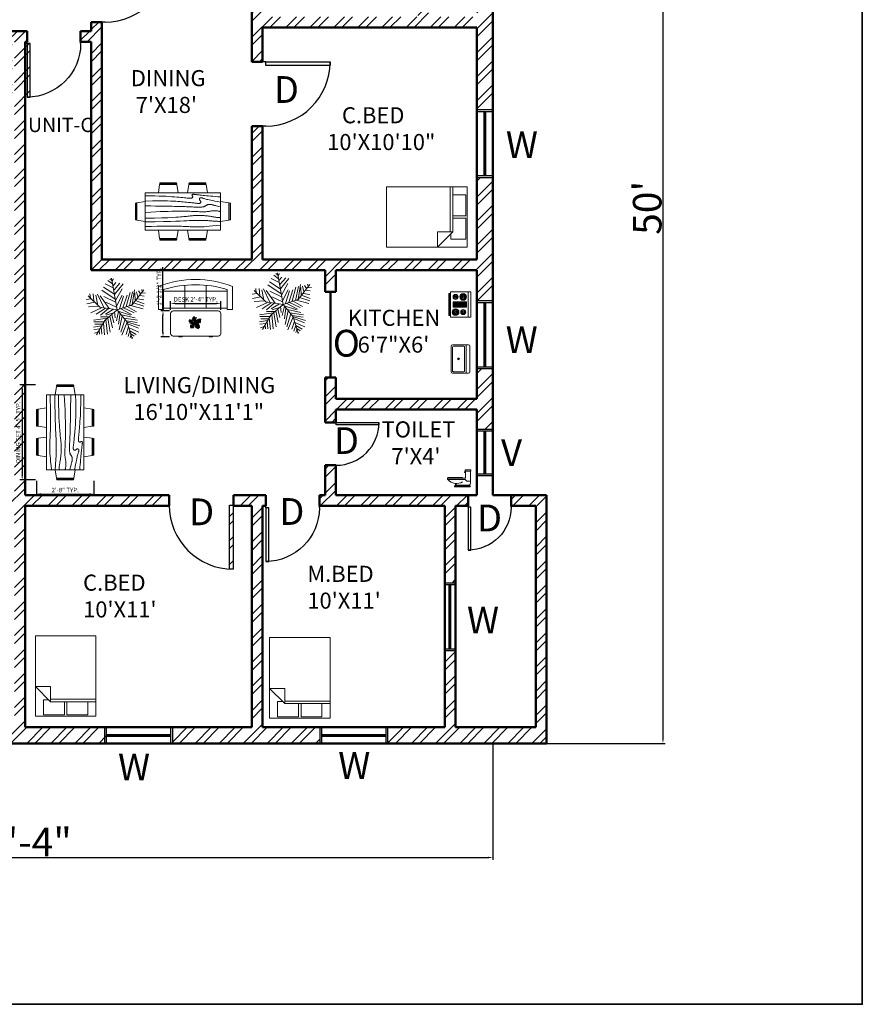
# Model space of a CAD drawing. Units: inches. Extents: x -31842 to -29388, y 18869 to 19743.
# Tile 11 of 12: x -29859 to -29388, y 18869 to 19420. Entities that reach past the tile are written whole.
import ezdxf

# ---------------------------------------------------------------- set-up
doc = ezdxf.new("R2010")
doc.units = ezdxf.units.IN
for name, color, linetype, lineweight in [('A-ANNO-DIMS', 2, 'Continuous', 18), ('A-ANNO-SYMB', 2, 'Continuous', 18), ('A-ANNO-TTLB', 7, 'Continuous', 35), ('A-AREA-IDEN', 3, 'Continuous', 18), ('A-DOOR', 3, 'Continuous', 25), ('A-FLOR-FIXT', 8, 'Continuous', 18), ('A-FURN', 8, 'Continuous', 18), ('A-GLAZ', 4, 'Continuous', 25), ('A-WALL', 7, 'Continuous', 50), ('A-WALL-PATT', 8, 'Continuous', 13), ('L-PLNT', 3, 'Continuous', 13)]:
    doc.layers.add(name, color=color, linetype=linetype, lineweight=lineweight)
doc.styles.get("Standard").update_dxf_attribs({"font": 'arial.ttf'})
doc.dimstyles.new('ISO-25', dxfattribs={"dimtxt": 2.5, "dimasz": 2.5, "dimexe": 1.25, "dimexo": 0.625, "dimtad": 1, "dimdec": 0, "dimlunit": 3, "dimtxsty": 'Standard', "dimcen": 2.5, "dimadec": 0, "dimazin": 0, "dimtfac": 1, "dimtdec": 0, "dimtmove": 0, "dimatfit": 3, "dimfxl": 1, "dimarcsym": 0})

# ---------------------------------------------------------------- blocks, each defined once
blk = doc.blocks.new('*U8')
for p, q in [((0, 0), (0, -100)), ((750, 0), (750, -100))]:
    blk.add_line(p, q)
blk.add_lwpolyline([(0, 0), (0, 750), (43.75, 750), (43.75, 0)], close=True)
blk.add_arc((0, 0), 750, 0, 90)
blk = doc.blocks.new('Bed - Queen')
for p, q in [((0, -80.00003), (0, 0)), ((0, 0), (59.99999, 0)), ((59.99999, 0), (59.99999, -80.00003)), ((7.99999, -1.2), (28.79998, -1.2)), ((7.99999, -14.4), (7.99999, -1.2)), ((28.79998, -1.2), (28.79998, -14.4)), ((31.19999, -1.2), (51.99999, -1.2)), ((31.19999, -14.4), (31.19999, -1.2)), ((51.99999, -1.2), (51.99999, -16.4)), ((0, -14.4), (44.8, -14.4)), ((44.8, -16.8), (0, -16.8)), ((59.99999, -29.6), (44.8, -14.4)), ((44.8, -14.4), (44.8, -29.6)), ((51.99999, -16.4), (46.79936, -16.4)), ((44.8, -29.6), (59.99999, -29.6)), ((59.99999, -80.00003), (0, -80.00003))]:
    blk.add_line(p, q)
blk = doc.blocks.new('Range-Oven - 30 in top')
for p, q in [((0, -3), (30, -3)), ((12, -6), (18, -6)), ((13, -20), (13, -6)), ((14, -6), (14, -20)), ((15, -20), (15, -6)), ((16, -6), (16, -20)), ((17, -20), (17, -6)), ((18, -20), (12, -20)), ((6, -24), (6, -25)), ((8, -25), (8, -24)), ((22, -25), (22, -24)), ((24, -24), (24, -25))]:
    blk.add_line(p, q)
for points in [[(0, -24), (0, 0), (30, 0), (30, -24)], [(12, -21), (12, -5), (18, -5), (18, -21)], [(2, -26), (2, -25), (28, -25), (28, -26)]]:
    blk.add_lwpolyline(points, close=True)
for centre, radius in [((6, -9), 4), ((6, -9), 3), ((6, -9), 2), ((6, -9), 1), ((24, -9), 3), ((24, -9), 2), ((24, -9), 1), ((6, -18), 3), ((6, -18), 2), ((6, -18), 1), ((24, -18), 4), ((24, -18), 3), ((24, -18), 2), ((24, -18), 1)]:
    blk.add_circle(centre, radius)
blk = doc.blocks.new('Sink-single - 30 in top')
blk.add_line((-15, -3.999996), (15, -3.999996))
for points in [[(-13.5, 0), (13.5, 0)], [(-15, -18.499996), (-15, -1.5)], [(-13.5, -17.499996), (-13.5, -6.499996)], [(-12.5, -5.499996), (12.5, -5.499996)], [(13.5, -6.499996), (13.5, -17.499996)], [(15, -1.5), (15, -18.499996)], [(13.5, -19.999996), (-13.5, -19.999996)], [(12.5, -18.499996), (-12.5, -18.499996)]]:
    blk.add_lwpolyline(points)
for radius in [1, 0.5]:
    blk.add_circle((0, -11.999996), radius)
for centre, radius, start, end in [((-13.5, -1.5), 1.5, 90, 180), ((-12.5, -6.499996), 1, 90, 180), ((12.5, -6.499996), 1, 0, 90), ((13.5, -1.5), 1.5, 0, 90), ((-13.5, -18.499996), 1.5, 180, 270), ((-12.5, -17.499996), 1, 180, 270), ((12.5, -17.499996), 1, 270, 0), ((13.5, -18.499996), 1.5, 270, 0)]:
    blk.add_arc(centre, radius, start, end)
blk = doc.blocks.new('Toilet - side')
for p, q in [((0.5, 5), (0.5, 22)), ((7.5, 22), (7.5, 12)), ((7.5, 21), (9, 21)), ((9, 20), (7.5, 20)), ((9, 21), (9, 20)), ((6, 8), (0.5, 8)), ((22, 2), (2, 2)), ((2, 2), (2, 1)), ((8, 10), (6, 8)), ((7.5, 12), (33, 12)), ((33, 10), (8, 10)), ((32.5, 13), (12, 13)), ((12, 13), (12, 12)), ((21, 4.5), (21, 2)), ((22, 2), (22, 4.5)), ((22, 1), (22, 2)), ((32.5, 12), (32.5, 13)), ((33, 12), (33, 10))]:
    blk.add_line(p, q)
for points in [[(0, 22), (0, 24), (8, 24), (8, 22)], [(1, 0), (1, 1), (23, 1), (23, 0)]]:
    blk.add_lwpolyline(points, close=True)
for centre, radius, start, end in [((3.8, 4.8), 3.26, 175.6013, 237.5288), ((20.3, 20.7), 16.2, 238.1872, 318.7702)]:
    blk.add_arc(centre, radius, start, end)
blk = doc.blocks.new('Desk - 30 x 60 in.')
for p, q in [((-26.999995, 0), (26.999995, 0)), ((-29.999995, -27), (-29.999995, -3)), ((29.999995, -3), (29.999995, -27)), ((26.999995, -30), (-26.999995, -30)), ((-20.000005, -30), (-20.000005, -31)), ((-20.000005, -31), (-16.000005, -31)), ((-16.000005, -31), (-16.000005, -30)), ((15.999995, -31), (15.999995, -30)), ((19.999995, -31), (15.999995, -31)), ((19.999995, -30), (19.999995, -31))]:
    blk.add_line(p, q)
for centre, start, end in [((-26.499995, -3.5), 98.1301, 171.8699), ((26.499995, -3.5), 8.130102, 81.8699), ((-26.499995, -26.5), 188.1301, 261.8699), ((26.499995, -26.5), 278.1301, 351.8699)]:
    blk.add_arc(centre, 3.535534, start, end)
blk = doc.blocks.new('Sofa - Roundback 7 ft.')
for p, q in [((-12.00002, -32.4421), (-12.00003, -6.5971)), ((11.99997, -32.4421), (11.99998, -6.5971)), ((-36.000027, -34), (-36.000027, -11.4696)), ((-35.999844, -13.3819), (35.9998, -13.3819)), ((35.99998, -34), (35.99998, -11.4696)), ((-36.000027, -32.4421), (35.99998, -32.4421))]:
    blk.add_line(p, q)
for points in [[(-36.000027, -34), (-42.000027, -34), (-42.000027, -8)], [(41.99998, -8), (41.99998, -34), (35.99998, -34)]]:
    blk.add_lwpolyline(points)
for centre, radius, start, end in [((0, -114.25), 114.25, 68.43141, 111.5686), ((-0.00001, -127.1968), 121.1968, 72.72033, 107.2797)]:
    blk.add_arc(centre, radius, start, end)
blk = doc.blocks.new('Dining Set - 36 x 72 in.')
for p, q in [((-22.2343, 26.00059), (-23.4847, 17.99762)), ((-22.2304, 26), (-5.7608, 26)), ((-22, 27.5), (-22.1562, 26.50042)), ((-5.8416, 26.5), (-22.1534, 26.5)), ((-22, 27.5), (-6, 27.5)), ((-5.8437, 26.49966), (-6, 27.5)), ((-4.5152, 17.99762), (-5.7655, 25.99926)), ((5.7657, 26.00059), (4.5153, 17.99762)), ((5.7696, 26), (22.2392, 26)), ((6, 27.5), (5.8438, 26.50042)), ((22.1584, 26.5), (5.8466, 26.5)), ((6, 27.5), (22, 27.5)), ((22.1563, 26.49966), (22, 27.5)), ((23.4848, 17.99762), (22.2345, 25.99926)), ((-44.0006, 8.23428), (-35.9976, 9.48474)), ((36, 18), (-36, 18)), ((-36, 18), (-36, -18)), ((44.0006, 8.23428), (35.9976, 9.48474)), ((36, -18), (36, 18)), ((-45.5, 8), (-44.5004, 8.15617)), ((-45.5, 8), (-45.5, -8)), ((-44.5, -8.15843), (-44.5, 8.15338)), ((-44, 8.23041), (-44, -8.23915)), ((44, 8.23041), (44, -8.23915)), ((44.5, -8.15843), (44.5, 8.15338)), ((45.5, 8), (44.5005, 8.15617)), ((45.5, 8), (45.5, -8)), ((-44.4997, -8.15631), (-45.5, -8)), ((-35.9976, -9.48476), (-43.9993, -8.2345)), ((35.9976, -9.48476), (43.9993, -8.2345)), ((44.4997, -8.15631), (45.5, -8)), ((-36, -18), (36, -18)), ((-22.2343, -26.0006), (-23.4847, -17.99762)), ((-4.5152, -17.99762), (-5.7655, -25.99928)), ((5.7657, -26.0006), (4.5153, -17.99762)), ((23.4848, -17.99762), (22.2345, -25.99928)), ((-22.2304, -26), (-5.7608, -26)), ((-22, -27.5), (-22.1562, -26.50044)), ((-5.8416, -26.5), (-22.1534, -26.5)), ((-22, -27.5), (-6, -27.5)), ((-5.8437, -26.49967), (-6, -27.5)), ((5.7696, -26), (22.2392, -26)), ((6, -27.5), (5.8438, -26.50044)), ((22.1584, -26.5), (5.8466, -26.5)), ((6, -27.5), (22, -27.5)), ((22.1563, -26.49967), (22, -27.5))]:
    blk.add_line(p, q)
for points in [[(-36, 15), (-31.1772, 14.97754), (-26.8079, 14.91406), (-22.8538, 14.81543), (-19.276, 14.6875), (-16.0362, 14.53613), (-13.0957, 14.36718), (-10.4159, 14.18652), (-7.9583, 14), (-5.6904, 13.81315), (-3.6035, 13.63021), (-1.6954, 13.45508), (0.0365, 13.29166), (1.5945, 13.14388), (2.9811, 13.01562), (4.1988, 12.9108), (5.25, 12.83333), (6.1393, 12.78613), (6.8802, 12.76823), (7.4883, 12.77767), (7.9792, 12.8125), (8.3685, 12.87077), (8.6719, 12.95052), (8.9049, 13.0498), (9.0833, 13.16666), (9.2205, 13.29899), (9.3216, 13.44401), (9.3895, 13.59879), (9.4271, 13.76041), (9.4373, 13.92594), (9.4232, 14.09245), (9.3875, 14.257), (9.3333, 14.41666), (9.2638, 14.56917), (9.1836, 14.71484), (9.0975, 14.85465), (9.0104, 14.98958), (8.9272, 15.1206), (8.8529, 15.2487), (8.7922, 15.37483), (8.75, 15.5), (8.7305, 15.62467), (8.7344, 15.74739), (8.7617, 15.86621), (8.8125, 15.97916), (8.8867, 16.08431), (8.9844, 16.17968), (9.1055, 16.26334), (9.25, 16.33333), (9.4189, 16.38802), (9.6172, 16.42708), (9.8506, 16.45052), (10.125, 16.45833), (10.4463, 16.45052), (10.8203, 16.42708), (11.2529, 16.38802), (11.75, 16.33333), (12.3184, 16.26318), (12.9694, 16.17838), (13.7151, 16.07991), (14.5677, 15.96875), (15.5395, 15.84586), (16.6426, 15.71224), (17.8893, 15.56884), (19.2917, 15.41666), (20.859, 15.25667), (22.5879, 15.08984), (24.4721, 14.91715), (26.5052, 14.73958), (28.6809, 14.5581), (30.9929, 14.3737), (33.4347, 14.18733), (36, 14)], [(-36, 10), (-28.9766, 10.14274), (-23.1725, 10.20442), (-18.4241, 10.19775), (-14.5677, 10.13541), (-11.4399, 10.03011), (-8.877, 9.89453), (-6.7154, 9.74137), (-4.7917, 9.58333), (-2.9698, 9.43082), (-1.2246, 9.28515), (0.4415, 9.14534), (2.026, 9.01041), (3.5266, 8.87939), (4.9408, 8.7513), (6.266, 8.62516), (7.5, 8.5), (8.6411, 8.37549), (9.6914, 8.2539), (10.6538, 8.13818), (11.5312, 8.03125), (12.3267, 7.93603), (13.043, 7.85547), (13.6831, 7.79248), (14.25, 7.75), (14.7471, 7.7303), (15.1797, 7.73307), (15.5537, 7.75732), (15.875, 7.80208), (16.1494, 7.86637), (16.3828, 7.94922), (16.5811, 8.04964), (16.75, 8.16666), (16.8944, 8.29915), (17.0143, 8.44531), (17.1089, 8.60319), (17.1771, 8.77083), (17.218, 8.94629), (17.2305, 9.1276), (17.2137, 9.31282), (17.1667, 9.5), (17.0895, 9.6875), (16.987, 9.875), (16.8649, 10.0625), (16.7292, 10.25), (16.5856, 10.4375), (16.4401, 10.625), (16.2985, 10.8125), (16.1667, 11), (16.05, 11.18733), (15.9518, 11.3737), (15.8752, 11.5581), (15.8229, 11.73958), (15.798, 11.91715), (15.8034, 12.08984), (15.842, 12.25667), (15.9167, 12.41666), (16.0295, 12.56836), (16.1784, 12.70833), (16.3605, 12.83268), (16.5729, 12.9375), (16.8127, 13.01888), (17.0768, 13.07291), (17.3625, 13.0957), (17.6667, 13.08333), (17.9894, 13.03312), (18.3418, 12.94726), (18.7382, 12.82918), (19.1927, 12.68229), (19.7195, 12.51001), (20.3327, 12.31575), (21.0465, 12.10294), (21.875, 11.875), (22.8357, 11.63354), (23.959, 11.37304), (25.2786, 11.08618), (26.8282, 10.76562), (28.6414, 10.40405), (30.752, 9.99414), (33.1936, 9.52856), (36, 9)], [(-36, 5.5), (-30.7157, 5.3348), (-26.069, 5.20963), (-21.9946, 5.11767), (-18.4271, 5.05208), (-15.3009, 5.00602), (-12.5508, 4.97265), (-10.1112, 4.94515), (-7.9167, 4.91666), (-5.909, 4.88167), (-4.0586, 4.83984), (-2.3429, 4.79215), (-0.7396, 4.73958), (0.7739, 4.6831), (2.22, 4.6237), (3.6213, 4.56233), (5, 4.5), (6.373, 4.43782), (7.7344, 4.3776), (9.0723, 4.32129), (10.375, 4.27083), (11.6309, 4.22819), (12.8281, 4.19531), (13.9551, 4.17415), (15, 4.16666), (15.954, 4.17448), (16.819, 4.19791), (17.6001, 4.23698), (18.3021, 4.29166), (18.9299, 4.36198), (19.4883, 4.44791), (19.9823, 4.54948), (20.4167, 4.66666), (20.7969, 4.79899), (21.1302, 4.94401), (21.4245, 5.09879), (21.6875, 5.26041), (21.9271, 5.42594), (22.1511, 5.59245), (22.3672, 5.757), (22.5834, 5.91666), (22.8065, 6.06868), (23.0404, 6.21093), (23.2879, 6.34147), (23.5521, 6.45833), (23.8358, 6.55957), (24.142, 6.64323), (24.4735, 6.70735), (24.8334, 6.75), (25.2235, 6.76969), (25.642, 6.76692), (26.0858, 6.74267), (26.5521, 6.69791), (27.0379, 6.63362), (27.5404, 6.55078), (28.0565, 6.45036), (28.5834, 6.33333), (29.1242, 6.19987), (29.7071, 6.04687), (30.3661, 5.87044), (31.1354, 5.66666), (32.0493, 5.43164), (33.142, 5.16146), (34.4475, 4.85221), (36, 4.5)], [(-36, -1), (-30.7915, -0.6591), (-26.0195, -0.38216), (-21.6519, -0.16284), (-17.6563, 0.00521), (-14.0005, 0.12833), (-10.6523, 0.21289), (-7.5796, 0.26522), (-4.75, 0.29166), (-2.134, 0.29793), (0.2878, 0.28711), (2.5317, 0.26163), (4.6146, 0.22396), (6.5529, 0.17651), (8.3633, 0.12174), (10.0623, 0.06209), (11.6667, 0), (13.1899, -0.06201), (14.6341, -0.1211), (15.9982, -0.17432), (17.2813, -0.21875), (18.4823, -0.25147), (19.6003, -0.26953), (20.6343, -0.27002), (21.5834, -0.25), (22.4481, -0.20768), (23.2357, -0.14584), (23.9549, -0.06836), (24.6146, 0.02083), (25.2235, 0.11784), (25.7904, 0.21875), (26.3241, 0.31966), (26.8334, 0.41666), (27.3265, 0.50618), (27.8099, 0.58593), (28.2894, 0.65397), (28.7709, 0.70833), (29.2601, 0.74707), (29.763, 0.76823), (30.2855, 0.76985), (30.8334, 0.75), (31.4088, 0.70784), (31.9994, 0.64713), (32.589, 0.57275), (33.1615, 0.48958), (33.7008, 0.4025), (34.1908, 0.3164), (34.6153, 0.23616), (34.9584, 0.16666), (35.2099, 0.11165), (35.3848, 0.07031), (35.504, 0.04069), (35.5886, 0.02083), (35.6594, 0.00879), (35.7377, 0.0026), (35.8442, 0.00032), (36, 0)], [(-36, -6.5), (-27.1843, -6.31267), (-20.084, -6.1263), (-14.469, -5.9419), (-10.1094, -5.76042), (-6.7752, -5.58285), (-4.2363, -5.41016), (-2.2629, -5.24333), (-0.625, -5.08334), (0.8708, -4.93099), (2.2715, -4.78646), (3.5872, -4.64974), (4.8281, -4.52084), (6.0046, -4.39974), (7.127, -4.28646), (8.2053, -4.18099), (9.25, -4.08334), (10.2705, -3.99382), (11.2734, -3.91407), (12.2647, -3.84603), (13.25, -3.79167), (14.2354, -3.75293), (15.2266, -3.73177), (16.2295, -3.73015), (17.25, -3.75), (18.2912, -3.79248), (19.3451, -3.85547), (20.4009, -3.93604), (21.4479, -4.03125), (22.4754, -4.13819), (23.4727, -4.25391), (24.4289, -4.37549), (25.3334, -4.5), (26.1785, -4.62492), (26.9694, -4.74935), (27.7145, -4.87281), (28.4219, -4.99479), (29.1, -5.11483), (29.7572, -5.23242), (30.4016, -5.34709), (31.0417, -5.45834), (31.6837, -5.56437), (32.3262, -5.65821), (32.9658, -5.73153), (33.599, -5.77604), (34.2224, -5.78345), (34.8327, -5.74545), (35.4264, -5.65373), (36, -5.5)], [(-36, -10), (-26.4022, -9.81299), (-18.4675, -9.62891), (-11.9839, -9.45069), (-6.7396, -9.28125), (-2.5226, -9.12354), (0.8789, -8.98047), (3.6769, -8.85498), (6.0833, -8.75), (8.2767, -8.66765), (10.3021, -8.60677), (12.1712, -8.56543), (13.8958, -8.54167), (15.4876, -8.53353), (16.9583, -8.53907), (18.3197, -8.55632), (19.5834, -8.58334), (20.7616, -8.61841), (21.8685, -8.66081), (22.9188, -8.71004), (23.9271, -8.76563), (24.9081, -8.82707), (25.8763, -8.89388), (26.8465, -8.96558), (27.8334, -9.04167), (28.8474, -9.12118), (29.8828, -9.20117), (30.93, -9.27824), (31.9792, -9.34896), (33.0205, -9.40991), (34.0443, -9.45768), (35.0407, -9.48885), (36, -9.5)], [(-36, -14.5), (-30.0881, -14.33513), (-25.0332, -14.21224), (-20.7312, -14.12647), (-17.0781, -14.07292), (-13.97, -14.04671), (-11.3027, -14.04297), (-8.9724, -14.05681), (-6.875, -14.08334), (-4.9224, -14.11833), (-3.0905, -14.16016), (-1.3709, -14.20785), (0.2448, -14.26042), (1.7647, -14.3169), (3.1973, -14.3763), (4.5507, -14.43767), (5.8333, -14.5), (7.0554, -14.5621), (8.235, -14.62175), (9.3922, -14.67652), (10.5469, -14.72396), (11.7192, -14.76164), (12.929, -14.78711), (14.1965, -14.79794), (15.5417, -14.79167), (16.9933, -14.76424), (18.6152, -14.70508), (20.4804, -14.60197), (22.6615, -14.44271), (25.2312, -14.21509), (28.2624, -13.9069), (31.8277, -13.50594), (36, -13)]]:
    blk.add_lwpolyline(points)
blk = doc.blocks.new('*U122')
for p, q in [((-258.7244, 1362.456), (-332.3336, 1421.4348)), ((0, 0), (-266.7, 1447.8)), ((-231.1146, 1315.2628), (-166.7002, 1421.4348)), ((-129.8956, 713.6638), (-626.7704, 1032.1544)), ((-185.1152, 1008.5578), (-553.1612, 1185.4942)), ((-221.9198, 1197.3052), (-433.5526, 1338.8594)), ((-194.31, 1102.9442), (-65.4812, 1256.284)), ((-148.3106, 914.1968), (118.5418, 1220.9018)), ((-129.8956, 701.8528), (265.7602, 1185.4942)), ((-74.7014, 418.7444), (219.7608, 961.39)), ((685.8, 228.6), (1219.2, 914.4)), ((689.0258, 230.0224), (790.2448, 914.1968)), ((1121.4862, 925.9824), (1149.0706, 831.6214)), ((-1206.4492, 501.3198), (-1418.082, 465.9376)), ((-800.1, 114.3), (-1333.5, 647.7)), ((-1234.059, 536.7274), (-1252.4486, 737.2604)), ((-1105.2302, 725.4494), (-1077.6458, 395.1732)), ((-976.4268, 666.4706), (-884.4026, 194.6402)), ((-902.8176, 713.6638), (-617.5756, 100.2538)), ((-369.1382, 53.086), (-783.1836, 642.874)), ((-93.091, 489.5342), (-700.3796, 902.3858)), ((-617.5756, 607.4918), (-74.7014, 347.98)), ((-28.6766, 171.0436), (228.9556, 678.2816)), ((100.1268, 41.275), (284.1498, 619.2774)), ((256.5654, 88.4682), (449.7832, 666.4706)), ((412.9786, 147.447), (587.8068, 796.2392)), ((560.197, 182.8292), (698.2206, 819.8358)), ((808.6344, 784.4282), (827.0494, 418.7444)), ((891.4384, 831.6214), (946.658, 572.1096)), ((919.0482, 501.3198), (1222.6798, 454.152)), ((983.4626, 867.0036), (1066.2666, 725.4494)), ((1029.462, 654.685), (1241.0948, 631.0884)), ((1112.2914, 760.8316), (1296.3144, 784.4282)), ((-1031.621, 347.98), (-1399.667, 277.1902)), ((-847.598, 159.2326), (-1326.0578, 135.636)), ((-718.7946, 88.4682), (-1215.644, -147.447)), ((-543.9664, 76.6572), (-967.2066, -206.4512)), ((0, 0), (-800.1, 114.3)), ((-405.9428, 53.086), (-764.794, -241.8334)), ((0, 0), (-571.5, -495.3)), ((-166.7002, 29.4894), (-543.9664, -206.4512)), ((-525.5514, 347.98), (-28.6766, 123.8504)), ((0, 0), (685.8, 228.6)), ((0, 0), (457.2, -571.5)), ((164.5412, 41.275), (661.416, -218.2368)), ((284.1498, 88.4682), (781.0246, -147.447)), ((458.978, 147.447), (891.4384, -88.4682)), ((615.4166, 194.6402), (1185.8752, 41.275)), ((753.4148, 312.5978), (1222.6798, 159.2326)), ((845.439, 418.7444), (1241.0948, 277.1902)), ((-442.7474, -383.3876), (-1086.8406, -477.7486)), ((-387.5278, -324.4088), (-764.794, -324.4088)), ((-166.7002, -147.447), (-507.1618, -253.619)), ((-433.5526, -383.3876), (-323.1134, -1020.3688)), ((-341.5284, -289.0012), (-221.9198, -831.6214)), ((-240.3094, -218.2368), (-157.5054, -595.7062)), ((-120.7008, -88.4682), (-93.091, -371.5766)), ((63.3222, -76.6826), (-37.8714, -513.1308)), ((44.9326, -64.897), (615.4166, -241.8334)), ((127.7366, -159.258), (54.1274, -654.685)), ((228.9556, -289.0012), (90.932, -914.1968)), ((357.759, -430.5554), (164.5412, -1020.3688)), ((192.151, -230.0224), (817.8292, -371.5766)), ((311.7596, -383.3876), (937.4378, -477.7486)), ((-718.7946, -737.2604), (-1086.8406, -796.2392)), ((-617.5756, -548.5384), (-1077.6458, -560.324)), ((-783.1836, -867.029), (-1077.6458, -902.4112)), ((-681.9646, -666.496), (-1022.4262, -654.685)), ((-571.5, -495.3), (-952.5, -1143)), ((-737.1842, -784.4536), (-709.5744, -1114.7298)), ((-635.9652, -607.5172), (-580.771, -1150.1374)), ((-525.5514, -465.963), (-451.9422, -1126.5408)), ((458.978, -572.1096), (210.5406, -1161.923)), ((514.1976, -772.6426), (403.7838, -1138.3264)), ((412.9786, -501.3452), (919.0482, -583.9206)), ((457.2, -571.5), (685.8, -1333.5)), ((468.1982, -572.1096), (1029.462, -737.2604)), ((486.5878, -642.8994), (983.4626, -843.4324)), ((541.8074, -831.6214), (992.6574, -1032.1544)), ((-875.2078, -1008.5832), (-1040.8412, -1079.3476)), ((-829.2084, -937.7934), (-810.7934, -1126.5408)), ((578.612, -961.39), (495.7826, -1232.7128)), ((578.612, -973.1756), (873.0488, -1138.3264)), ((624.6114, -1161.923), (587.8068, -1291.6916)), ((624.6114, -1102.9442), (781.0246, -1209.1162)), ((679.8056, -1268.095), (716.6102, -1291.6916))]:
    blk.add_line(p, q)
blk = doc.blocks.new('*D211')
at = {"layer": 'A-ANNO-DIMS', "color": 0, "lineweight": -2, "transparency": 16777216}
for p, q in [((-29593.87, 19614.96), (-29498.06, 19614.96)), ((-29499.31, 19612.46), (-29499.31, 19017.46)), ((-29593.87, 19014.96), (-29498.06, 19014.96))]:
    blk.add_line(p, q, dxfattribs=at)
at = {"layer": 'A-ANNO-DIMS', "color": 0, "transparency": 16777216}
for points in [[(-29499.72, 19612.46), (-29498.89, 19612.46), (-29499.31, 19614.96)], [(-29499.72, 19017.46), (-29498.89, 19017.46), (-29499.31, 19014.96)]]:
    blk.add_solid(points, dxfattribs=at)
at = {"layer": 'Defpoints', "color": 0, "transparency": 16777216}
for p in [(-29594.5, 19614.96), (-29594.5, 19014.96), (-29499.31, 19014.96)]:
    blk.add_point(p, dxfattribs=at)
at = {"layer": 'A-ANNO-DIMS', "color": 0, "transparency": 16777216, "insert": (-29508.1, 19314.96), "char_height": 2.5, "attachment_point": 5, "rotation": 90}
blk.add_mtext("{\\H6.4x;50'}", dxfattribs=at)
blk = doc.blocks.new('*D212')
at = {"layer": 'A-ANNO-DIMS', "color": 0, "lineweight": -2, "transparency": 16777216}
for p, q in [((-30126.5, 19014.34), (-30126.5, 18949.8)), ((-29594.5, 19014.34), (-29594.5, 18949.8)), ((-30124, 18951.05), (-29597, 18951.05))]:
    blk.add_line(p, q, dxfattribs=at)
at = {"layer": 'A-ANNO-DIMS', "color": 0, "transparency": 16777216}
for points in [[(-30124, 18951.47), (-30124, 18950.64), (-30126.5, 18951.05)], [(-29597, 18951.47), (-29597, 18950.64), (-29594.5, 18951.05)]]:
    blk.add_solid(points, dxfattribs=at)
at = {"layer": 'Defpoints', "color": 0, "transparency": 16777216}
for p in [(-30126.5, 19014.96), (-29594.5, 19014.96), (-29594.5, 18951.05)]:
    blk.add_point(p, dxfattribs=at)
at = {"layer": 'A-ANNO-DIMS', "color": 0, "transparency": 16777216, "insert": (-29860.5, 18959.68), "char_height": 2.5, "attachment_point": 5}
blk.add_mtext('{\\H6.4x;44\'-4"}', dxfattribs=at)
blk = doc.blocks.new('WIN-3FT')
for p, q in [((0, 36), (9, 36)), ((4, 0), (4, 36)), ((4.5, 0), (4.5, 36)), ((5, 0), (5, 36)), ((0, 0), (9, 0))]:
    blk.add_line(p, q)
blk = doc.blocks.new('WIN-3FT-B')
for p, q in [((0, 36), (6, 36)), ((2.5, 0), (2.5, 36)), ((3, 0), (3, 36)), ((3.5, 0), (3.5, 36)), ((0, 0), (6, 0))]:
    blk.add_line(p, q)
blk = doc.blocks.new('WIN-2FT')
for p, q in [((0, 24), (9, 24)), ((4, 0), (4, 24)), ((4.5, 0), (4.5, 24)), ((5, 0), (5, 24)), ((0, 0), (9, 0))]:
    blk.add_line(p, q)
blk = doc.blocks.new('*D245')
at = {"layer": 'A-ANNO-DIMS', "color": 0, "lineweight": -2, "transparency": 16777216}
for p, q in [((-29850.74, 19215.8), (-29859.34, 19215.8)), ((-29858.09, 19213.3), (-29858.09, 19165.11)), ((-29850.74, 19162.61), (-29859.34, 19162.61))]:
    blk.add_line(p, q, dxfattribs=at)
at = {"layer": 'A-ANNO-DIMS', "color": 0, "transparency": 16777216}
for points in [[(-29858.51, 19213.3), (-29857.67, 19213.3), (-29858.09, 19215.8)], [(-29858.51, 19165.11), (-29857.67, 19165.11), (-29858.09, 19162.61)]]:
    blk.add_solid(points, dxfattribs=at)
at = {"layer": 'Defpoints', "color": 0, "transparency": 16777216}
for p in [(-29850.11, 19215.8), (-29858.09, 19162.61), (-29850.11, 19162.61)]:
    blk.add_point(p, dxfattribs=at)
at = {"layer": 'A-ANNO-DIMS', "color": 0, "transparency": 16777216, "insert": (-29860.01, 19189.21), "char_height": 2.5, "attachment_point": 5, "rotation": 90}
blk.add_mtext('DINING SET 4\'-5" TYP.', dxfattribs=at)
blk = doc.blocks.new('*D246')
at = {"layer": 'A-ANNO-DIMS', "color": 0, "lineweight": -2, "transparency": 16777216}
for p, q in [((-29850.11, 19161.98), (-29850.11, 19153.38)), ((-29817.96, 19161.98), (-29817.96, 19153.38)), ((-29847.61, 19154.63), (-29820.46, 19154.63))]:
    blk.add_line(p, q, dxfattribs=at)
at = {"layer": 'A-ANNO-DIMS', "color": 0, "transparency": 16777216}
for points in [[(-29847.61, 19155.04), (-29847.61, 19154.21), (-29850.11, 19154.63)], [(-29820.46, 19155.04), (-29820.46, 19154.21), (-29817.96, 19154.63)]]:
    blk.add_solid(points, dxfattribs=at)
at = {"layer": 'Defpoints', "color": 0, "transparency": 16777216}
for p in [(-29850.11, 19162.61), (-29817.96, 19162.61), (-29817.96, 19154.63)]:
    blk.add_point(p, dxfattribs=at)
at = {"layer": 'A-ANNO-DIMS', "color": 0, "transparency": 16777216, "insert": (-29834.03, 19156.53), "char_height": 2.5, "attachment_point": 5}
blk.add_mtext('2\'-8" TYP.', dxfattribs=at)
blk = doc.blocks.new('*D251')
at = {"layer": 'A-ANNO-DIMS', "color": 0, "lineweight": -2, "transparency": 16777216}
for p, q in [((-29775.03, 19257.82), (-29775.03, 19262.67)), ((-29772.53, 19261.42), (-29749.36, 19261.42)), ((-29746.86, 19257.82), (-29746.86, 19262.67))]:
    blk.add_line(p, q, dxfattribs=at)
at = {"layer": 'A-ANNO-DIMS', "color": 0, "transparency": 16777216}
for points in [[(-29772.53, 19261.84), (-29772.53, 19261.01), (-29775.03, 19261.42)], [(-29749.36, 19261.84), (-29749.36, 19261.01), (-29746.86, 19261.42)]]:
    blk.add_solid(points, dxfattribs=at)
at = {"layer": 'Defpoints', "color": 0, "transparency": 16777216}
for p in [(-29746.86, 19261.42), (-29775.03, 19257.2), (-29746.86, 19257.2)]:
    blk.add_point(p, dxfattribs=at)
at = {"layer": 'A-ANNO-DIMS', "color": 0, "transparency": 16777216, "insert": (-29760.95, 19263.34), "char_height": 2.5, "attachment_point": 5}
blk.add_mtext('DESK 2\'-4" TYP.', dxfattribs=at)
blk = doc.blocks.new('*D252')
at = {"layer": 'A-ANNO-DIMS', "color": 0, "lineweight": -2, "transparency": 16777216}
for p, q in [((-29779.26, 19257.2), (-29779.26, 19281.78)), ((-29775.66, 19257.2), (-29780.51, 19257.2)), ((-29779.26, 19245.14), (-29779.26, 19254.7)), ((-29775.66, 19242.64), (-29780.51, 19242.64))]:
    blk.add_line(p, q, dxfattribs=at)
at = {"layer": 'A-ANNO-DIMS', "color": 0, "transparency": 16777216}
for points in [[(-29779.68, 19254.7), (-29778.84, 19254.7), (-29779.26, 19257.2)], [(-29779.68, 19245.14), (-29778.84, 19245.14), (-29779.26, 19242.64)]]:
    blk.add_solid(points, dxfattribs=at)
at = {"layer": 'Defpoints', "color": 0, "transparency": 16777216}
for p in [(-29779.26, 19257.2), (-29775.03, 19257.2), (-29775.03, 19242.64)]:
    blk.add_point(p, dxfattribs=at)
at = {"layer": 'A-ANNO-DIMS', "color": 0, "transparency": 16777216, "insert": (-29781.18, 19270.74), "char_height": 2.5, "attachment_point": 5, "rotation": 90}
blk.add_mtext('1\'-2 1/2" TYP.', dxfattribs=at)

msp = doc.modelspace()

# ---------------------------------------------------------------- hatches: boundary and pattern name
at = {"layer": 'A-WALL-PATT'}
h = msp.add_hatch(dxfattribs=at)
h.set_pattern_fill('ANSI32', color=256)
h.paths.add_polyline_path([(-29790.5, 19614.96), (-29841.5, 19614.96), (-29841.5, 19605.96), (-29819.5, 19605.96), (-29819.5, 19455.01), (-29813.5, 19455.01), (-29813.5, 19491.96), (-29800.11, 19491.96), (-29800.11, 19497.96), (-29813.5, 19497.96), (-29813.5, 19605.96), (-29790.5, 19605.96)])
h.paths.add_polyline_path([(-29879.5, 19614.96), (-29930.5, 19614.96), (-29930.5, 19605.96), (-29907.5, 19605.96), (-29907.5, 19497.96), (-29922.61, 19497.96), (-29922.61, 19491.96), (-29907.5, 19491.96), (-29907.5, 19456.33), (-29903.21, 19456.33), (-29901.5, 19456.31), (-29901.5, 19605.96), (-29879.5, 19605.96)])
h.paths.add_polyline_path([(-29968.5, 19614.96), (-29991.5, 19614.96), (-29991.5, 19656.96), (-30126.5, 19656.96), (-30126.5, 19559.96), (-30117.5, 19559.96), (-30117.5, 19605.96), (-30029.48, 19605.96), (-30029.48, 19614.96), (-30117.5, 19614.96), (-30117.5, 19650.96), (-29997.5, 19650.96), (-29997.5, 19614.96), (-30005.48, 19614.96), (-30005.48, 19605.96), (-29997.5, 19605.96), (-29997.5, 19549.04), (-29991.5, 19549.04), (-29991.5, 19605.96), (-29968.5, 19605.96)])
h.paths.add_polyline_path([(-29716.42, 19614.96), (-29723.5, 19614.96), (-29723.5, 19650.96), (-29603.5, 19650.96), (-29603.5, 19614.96), (-29692.42, 19614.96), (-29692.42, 19605.96), (-29687.14, 19605.96), (-29603.5, 19605.96), (-29603.5, 19559.96), (-29594.5, 19559.96), (-29594.5, 19656.96), (-29729.5, 19656.96), (-29729.5, 19614.96), (-29752.5, 19614.96), (-29752.5, 19605.96), (-29729.5, 19605.96), (-29729.5, 19551.13), (-29723.5, 19551.13), (-29723.5, 19605.96), (-29716.42, 19605.96)])
h.paths.add_polyline_path([(-29628.39, 19472.82), (-29628.34, 19475.96), (-29723.5, 19475.96), (-29723.5, 19515.13), (-29729.5, 19515.13), (-29729.5, 19497.96), (-29744.93, 19497.96), (-29744.93, 19491.96), (-29729.5, 19491.96), (-29729.5, 19460.98), (-29723.5, 19460.98), (-29723.5, 19469.96), (-29636.5, 19469.96), (-29636.5, 19458.96), (-29630.5, 19458.96), (-29630.5, 19469.96), (-29628.39, 19469.96)])
h.paths.add_polyline_path([(-29594.5, 19521.96), (-29603.5, 19521.96), (-29603.5, 19475.96), (-29604.34, 19475.96), (-29604.34, 19469.96), (-29603.5, 19469.96), (-29603.5, 19421.96), (-29630.5, 19421.96), (-29630.5, 19432.96), (-29636.5, 19432.96), (-29636.5, 19421.96), (-29723.5, 19421.96), (-29723.5, 19436.98), (-29729.5, 19436.98), (-29729.5, 19396.75), (-29723.5, 19396.75), (-29723.5, 19415.96), (-29603.5, 19415.96), (-29603.5, 19369.96), (-29594.5, 19369.96)])
h.paths.add_polyline_path([(-29594.5, 19331.96), (-29603.5, 19331.96), (-29603.5, 19285.96), (-29723.5, 19285.96), (-29723.5, 19360.75), (-29729.5, 19360.75), (-29729.5, 19285.96), (-29813.5, 19285.96), (-29813.5, 19419.01), (-29819.5, 19419.01), (-29819.5, 19413.96), (-29825.38, 19413.96), (-29825.38, 19407.96), (-29819.5, 19407.96), (-29819.5, 19279.96), (-29688.5, 19279.96), (-29688.5, 19267.87), (-29682.5, 19267.87), (-29682.5, 19279.96), (-29603.5, 19279.96), (-29603.5, 19262.96), (-29594.5, 19262.96)])
h.paths.add_polyline_path([(-29594.5, 19224.96), (-29603.5, 19224.96), (-29603.5, 19207.96), (-29682.5, 19207.96), (-29682.5, 19219.98), (-29688.5, 19219.98), (-29688.5, 19194.76), (-29682.5, 19194.76), (-29682.5, 19201.96), (-29603.5, 19201.96), (-29603.5, 19190.96), (-29594.5, 19190.96)])
h.paths.add_polyline_path([(-29564.5, 19153.96), (-29584.31, 19153.96), (-29584.31, 19147.96), (-29570.5, 19147.96), (-29570.5, 19023.96), (-29615.5, 19023.96), (-29615.5, 19066.96), (-29621.5, 19066.96), (-29621.5, 19023.96), (-29653.5, 19023.96), (-29653.5, 19014.96), (-29564.5, 19014.96)])
h.paths.add_polyline_path([(-29608.31, 19153.96), (-29682.5, 19153.96), (-29682.5, 19170.76), (-29688.5, 19170.76), (-29688.5, 19153.96), (-29691.71, 19153.96), (-29691.71, 19147.96), (-29621.5, 19147.96), (-29621.5, 19104.96), (-29615.5, 19104.96), (-29615.5, 19147.96), (-29608.31, 19147.96)])
h.paths.add_polyline_path([(-29721.71, 19153.96), (-29739.81, 19153.96), (-29739.81, 19147.96), (-29729.5, 19147.96), (-29729.5, 19023.96), (-29774, 19023.96), (-29774, 19014.96), (-29691.5, 19014.96), (-29691.5, 19023.96), (-29723.5, 19023.96), (-29723.5, 19147.96), (-29721.71, 19147.96)])
h.paths.add_polyline_path([(-29946, 19023.96), (-29991.5, 19023.96), (-29991.5, 19147.96), (-29988.28, 19147.96), (-29988.28, 19153.96), (-30000.21, 19153.96), (-30000.21, 19147.96), (-29997.5, 19147.96), (-29997.5, 19023.96), (-30029.5, 19023.96), (-30029.5, 19014.96), (-29946, 19014.96)])
h.paths.add_polyline_path([(-30067.5, 19023.96), (-30099.5, 19023.96), (-30099.5, 19066.96), (-30105.5, 19066.96), (-30105.5, 19023.96), (-30150.5, 19023.96), (-30150.5, 19147.96), (-30137.18, 19147.96), (-30137.18, 19153.96), (-30156.5, 19153.96), (-30156.5, 19014.96), (-30067.5, 19014.96)])
h.paths.add_polyline_path([(-30099.5, 19147.96), (-30030.21, 19147.96), (-30030.21, 19153.96), (-30032.5, 19153.96), (-30032.5, 19173.83), (-30038.5, 19173.83), (-30038.5, 19153.96), (-30113.18, 19153.96), (-30113.18, 19147.96), (-30105.5, 19147.96), (-30105.5, 19104.96), (-30099.5, 19104.96)])
h.paths.add_polyline_path([(-30032.5, 19217.89), (-30038.5, 19217.89), (-30038.5, 19207.96), (-30117.5, 19207.96), (-30117.5, 19224.96), (-30126.5, 19224.96), (-30126.5, 19190.96), (-30117.5, 19190.96), (-30117.5, 19201.96), (-30038.5, 19201.96), (-30038.5, 19197.83), (-30032.5, 19197.83)])
h.paths.add_polyline_path([(-29901.5, 19407.96), (-29893.72, 19407.96), (-29893.72, 19413.96), (-29901.5, 19413.96), (-29901.5, 19420.31), (-29907.5, 19420.31), (-29907.5, 19285.96), (-29991.5, 19285.96), (-29991.5, 19365.01), (-29997.5, 19365.01), (-29997.5, 19285.96), (-30117.5, 19285.96), (-30117.5, 19331.96), (-30126.5, 19331.96), (-30126.5, 19262.96), (-30117.5, 19262.96), (-30117.5, 19279.96), (-30038.5, 19279.96), (-30038.5, 19268.29), (-30032.5, 19268.29), (-30032.5, 19279.96), (-29901.5, 19279.96)])
h.paths.add_polyline_path([(-29863.72, 19413.96), (-29855.38, 19413.96), (-29855.38, 19406.96), (-29853.63, 19406.96), (-29853.63, 19376.96), (-29856.5, 19376.96), (-29856.5, 19153.96), (-29775.81, 19153.96), (-29775.81, 19148.44, 0.39722), (-29741.97, 19112.57), (-29741.97, 19148.44), (-29739.88, 19148.44), (-29739.88, 19112.51), (-29741.97, 19112.51), (-29741.97, 19112.57, -0.393359), (-29775.8, 19147.96), (-29856.5, 19147.96), (-29856.5, 19023.96), (-29811, 19023.96), (-29811, 19014.96), (-29909, 19014.96), (-29909, 19018.96), (-29945, 19018.96), (-29945, 19019.96), (-29909, 19019.96), (-29909, 19023.96), (-29862.5, 19023.96), (-29862.5, 19147.96), (-29901.5, 19147.96), (-29952.22, 19147.96), (-29952.22, 19146.6, -0.39722), (-29986.12, 19110.67), (-29986.12, 19110.6), (-29988.22, 19110.6), (-29988.22, 19146.6), (-29986.12, 19146.6), (-29986.12, 19110.67, 0.39722), (-29952.22, 19146.6), (-29952.22, 19147.96), (-29952.28, 19147.96), (-29952.28, 19153.96), (-29901.5, 19153.96), (-29862.5, 19153.96), (-29862.5, 19407.96), (-29863.72, 19407.96), (-29863.72, 19406.62), (-29863.72, 19376.63), (-29865.47, 19376.63), (-29865.47, 19406.62), (-29863.72, 19406.62), (-29863.72, 19407.96), (-29863.72, 19407.96)])
h.paths.add_polyline_path([(-30021.02, 19461.17), (-30021.06, 19461.17), (-30021.06, 19462.57), (-29997.02, 19462.57), (-29997.02, 19461.17), (-30021.02, 19461.17, 0.386026), (-29997.95, 19438.55), (-29991.5, 19438.55), (-29991.5, 19401.01), (-29998.66, 19401.01), (-29998.66, 19398.9), (-30034.72, 19398.9), (-30034.72, 19401.01), (-29997.5, 19401.01), (-29997.5, 19415.96), (-30117.5, 19415.96), (-30117.5, 19368.96), (-30121.5, 19368.96), (-30121.5, 19332.96), (-30122.5, 19332.96), (-30122.5, 19368.96), (-30126.5, 19368.96), (-30126.5, 19522.96), (-30117.5, 19522.96), (-30117.5, 19475.96), (-30116.52, 19475.96), (-30116.52, 19469.92, 0.39722), (-30093.92, 19445.96), (-30093.92, 19469.92), (-30092.52, 19469.92), (-30092.52, 19445.92), (-30093.92, 19445.92), (-30093.92, 19445.96, -0.39722), (-30116.52, 19469.92), (-30117.5, 19421.96), (-30090.5, 19421.96), (-30090.5, 19433.96), (-30084.5, 19433.96), (-30084.5, 19421.96), (-29997.5, 19421.96), (-29997.5, 19438.54, -0.391477)])
h.paths.add_polyline_path([(-29991.5, 19491.96), (-29980.66, 19491.96), (-29980.66, 19497.96), (-29991.5, 19497.96), (-29991.5, 19513.04), (-29997.5, 19513.04), (-29997.5, 19475.96), (-30092.52, 19475.96), (-30092.52, 19469.96), (-30090.5, 19469.96), (-30090.5, 19458.96), (-30084.5, 19458.96), (-30084.5, 19469.96), (-29997.5, 19469.96), (-29997.5, 19462.57), (-29997.02, 19462.57), (-29991.5, 19462.55)])
h.paths.add_polyline_path([(-29857.76, 19352.86), (-29815.8, 19352.86), (-29815.8, 19369.38), (-29857.76, 19369.38)], flags=24)

# ---------------------------------------------------------------- linework, layer by layer
at = {"layer": 'A-ANNO-TTLB'}
msp.add_lwpolyline([(-31842.18, 19743.36), (-29387.67, 19743.36), (-29387.67, 18868.82), (-31842.18, 18868.82)], close=True, dxfattribs=at)
at = {"layer": 'A-GLAZ'}
for p, q in [((-29603.5, 19369.96), (-29594.5, 19369.96)), ((-29603.5, 19331.96), (-29594.5, 19331.96)), ((-29603.5, 19262.96), (-29594.5, 19262.96)), ((-29603.5, 19224.96), (-29594.5, 19224.96)), ((-29603.5, 19190.96), (-29594.5, 19190.96)), ((-29603.5, 19164.96), (-29594.5, 19164.96)), ((-29621.5, 19104.96), (-29615.5, 19104.96)), ((-29621.5, 19066.96), (-29615.5, 19066.96)), ((-29812, 19023.96), (-29812, 19014.96)), ((-29774, 19023.96), (-29774, 19014.96)), ((-29691.5, 19023.96), (-29691.5, 19014.96)), ((-29653.5, 19023.96), (-29653.5, 19014.96))]:
    msp.add_line(p, q, dxfattribs=at)
at = {"layer": 'A-WALL'}
for p, q in [((-29594.5, 19656.96), (-29594.5, 19153.96)), ((-29729.5, 19436.98), (-29729.5, 19396.75)), ((-29819.5, 19419.01), (-29813.5, 19419.01)), ((-29819.5, 19419.01), (-29819.5, 19413.96)), ((-29813.5, 19419.01), (-29813.5, 19285.96)), ((-29863.72, 19413.96), (-29855.38, 19413.96)), ((-29855.38, 19407.96), (-29855.38, 19413.96)), ((-29825.38, 19407.96), (-29825.38, 19413.96)), ((-29825.38, 19413.96), (-29819.5, 19413.96)), ((-29723.5, 19415.96), (-29603.5, 19415.96)), ((-29723.5, 19415.96), (-29723.5, 19396.75)), ((-29603.5, 19415.96), (-29603.5, 19285.96)), ((-29856.5, 19153.96), (-29856.5, 19407.96)), ((-29856.5, 19407.96), (-29855.38, 19407.96)), ((-29825.38, 19407.96), (-29819.5, 19407.96)), ((-29819.5, 19407.96), (-29819.5, 19279.96)), ((-29729.5, 19396.75), (-29723.5, 19396.75)), ((-29729.5, 19360.75), (-29723.5, 19360.75)), ((-29729.5, 19360.75), (-29729.5, 19285.96)), ((-29723.5, 19360.75), (-29723.5, 19285.96)), ((-29813.5, 19285.96), (-29729.5, 19285.96)), ((-29723.5, 19285.96), (-29603.5, 19285.96)), ((-29819.5, 19279.96), (-29688.5, 19279.96)), ((-29688.5, 19279.96), (-29688.5, 19267.87)), ((-29682.5, 19279.96), (-29682.5, 19267.87)), ((-29682.5, 19279.96), (-29603.5, 19279.96)), ((-29603.5, 19279.96), (-29603.5, 19207.96)), ((-29688.5, 19267.87), (-29682.5, 19267.87)), ((-29685.5, 19267.87), (-29685.5, 19219.98)), ((-29688.5, 19219.98), (-29682.5, 19219.98)), ((-29688.5, 19219.98), (-29688.5, 19194.76)), ((-29682.5, 19219.98), (-29682.5, 19207.96)), ((-29682.5, 19207.96), (-29603.5, 19207.96)), ((-29682.5, 19201.96), (-29603.5, 19201.96)), ((-29682.5, 19201.96), (-29682.5, 19194.76)), ((-29603.5, 19201.96), (-29603.5, 19153.96)), ((-29688.5, 19194.76), (-29682.5, 19194.76)), ((-29688.5, 19170.76), (-29682.5, 19170.76)), ((-29688.5, 19170.76), (-29688.5, 19153.96)), ((-29682.5, 19170.76), (-29682.5, 19153.96)), ((-29856.5, 19153.96), (-29775.81, 19153.96)), ((-29775.81, 19147.96), (-29775.81, 19153.96)), ((-29739.81, 19147.96), (-29739.81, 19153.96)), ((-29739.81, 19153.96), (-29721.71, 19153.96)), ((-29721.71, 19153.96), (-29721.71, 19147.96)), ((-29691.71, 19153.96), (-29691.71, 19147.96)), ((-29691.71, 19153.96), (-29688.5, 19153.96)), ((-29682.5, 19153.96), (-29603.5, 19153.96)), ((-29608.31, 19153.96), (-29608.31, 19147.96)), ((-29594.5, 19153.96), (-29564.5, 19153.96)), ((-29584.31, 19153.96), (-29584.31, 19147.96)), ((-29564.5, 19153.96), (-29564.5, 19014.96)), ((-29856.5, 19023.96), (-29856.5, 19147.96)), ((-29856.5, 19147.96), (-29775.81, 19147.96)), ((-29739.81, 19147.96), (-29729.5, 19147.96)), ((-29729.5, 19147.96), (-29729.5, 19023.96)), ((-29723.5, 19147.96), (-29723.5, 19023.96)), ((-29723.5, 19147.96), (-29721.71, 19147.96)), ((-29691.71, 19147.96), (-29621.5, 19147.96)), ((-29621.5, 19147.96), (-29621.5, 19023.96)), ((-29615.5, 19147.96), (-29615.5, 19023.96)), ((-29615.5, 19147.96), (-29608.31, 19147.96)), ((-29584.31, 19147.96), (-29570.5, 19147.96)), ((-29570.5, 19147.96), (-29570.5, 19023.96)), ((-29729.5, 19023.96), (-29856.5, 19023.96)), ((-29621.5, 19023.96), (-29723.5, 19023.96)), ((-29570.5, 19023.96), (-29615.5, 19023.96)), ((-29564.5, 19014.96), (-30156.5, 19014.96))]:
    msp.add_line(p, q, dxfattribs=at)

# ---------------------------------------------------------------- block references
at = {"layer": 'A-DOOR'}
for p, xscale, yscale, zscale, rotation in [((-29811.71, 19454.93), 0.0478936875771185, 0.0478936875771185, 0.0478936875771185, 270), ((-29855.38, 19406.96), -0.0399999999999929, 0.0399999999999929, 0.0399999999999929, 180), ((-29721.7, 19396.75), 0.0479999986246562, 0.0479999986246562, 0.0479999986246562, 270), ((-29682.3, 19194.76), 0.0320000009996835, 0.0320000009996835, 0.0320000009996835, 270), ((-29739.88, 19148.44), 0.0479065092540991, 0.0479065092540991, 0.0479065092540991, 180), ((-29721.7, 19146.88), -0.0399999999999929, 0.0399999999999929, 0.0399999999999929, 180), ((-29608.34, 19147.32), -0.0320770016506898, 0.0320770016506898, 0.0320770016506898, 180)]:
    msp.add_blockref('*U8', p, dxfattribs=dict(at, xscale=xscale, yscale=yscale, zscale=zscale, rotation=rotation))
at = {"layer": 'A-FLOR-FIXT', "rotation": 270}
for name, p, xscale, yscale, zscale in [('Range-Oven - 30 in top', (-29606.9, 19267.86), 0.4722739601602511, 0.4722739601602511, 0.4722739601602511), ('Sink-single - 30 in top', (-29607.44, 19230.27), 0.526605956738203, 0.526605956738203, 0.526605956738203)]:
    msp.add_blockref(name, p, dxfattribs=dict(at, xscale=xscale, yscale=yscale, zscale=zscale))
at = {"layer": 'A-FLOR-FIXT', "xscale": -0.3964966977869737, "yscale": 0.3964966977869737, "zscale": 0.3964966977869737}
msp.add_blockref('Toilet - side', (-29606.82, 19158.75), dxfattribs=at)
at = {"layer": 'A-FURN'}
for name, p, xscale, yscale, zscale in [('Dining Set - 36 x 72 in.', (-29768.13, 19312.89), 0.5845828142739601, 0.5845828142739601, 0.5845828142739601), ('Sofa - Roundback 7 ft.', (-29761.06, 19274.85), 0.4950711502487754, 0.4950711502487754, 0.4950711502487754), ('Desk - 30 x 60 in.', (-29760.95, 19257.2), 0.4695867386829459, 0.4695867386829459, 0.4695867386829459)]:
    msp.add_blockref(name, p, dxfattribs=dict(at, xscale=xscale, yscale=yscale, zscale=zscale))
for name, p, xscale, yscale, zscale, rotation in [('Bed - Queen', (-29608.91, 19326.77), 0.5638390730281776, 0.5638390730281776, 0.5638390730281776, 270), ('Dining Set - 36 x 72 in.', (-29834.03, 19189.21), 0.5845828142739601, 0.5845828142739601, 0.5845828142739601, 270), ('Bed - Queen', (-29816.9, 19030.19), 0.5638390730281776, 0.5638390730281776, 0.5638390730281776, 180), ('Bed - Queen', (-29685.73, 19029.11), 0.5638390730281776, 0.5638390730281776, 0.5638390730281776, 180)]:
    msp.add_blockref(name, p, dxfattribs=dict(at, xscale=xscale, yscale=yscale, zscale=zscale, rotation=rotation))
at = {"layer": 'A-GLAZ'}
for name, p in [('WIN-3FT', (-29603.5, 19332.96)), ('WIN-3FT', (-29603.5, 19225.96)), ('WIN-2FT', (-29603.5, 19165.96)), ('WIN-3FT-B', (-29621.5, 19067.96))]:
    msp.add_blockref(name, p, dxfattribs=at)
at = {"layer": 'A-GLAZ', "rotation": 269.9999999999782}
for p in [(-29811, 19023.96), (-29690.5, 19023.96)]:
    msp.add_blockref('WIN-3FT', p, dxfattribs=at)
at = {"layer": 'L-PLNT'}
for p, xscale, yscale, zscale in [((-29804.88, 19257.83), 0.0122024487722625, 0.0122024487722625, 0.0122024487722625), ((-29711.97, 19260.82), 0.0122024487722625, 0.0122024487722625, 0.0122024487722625), ((-29761.23, 19250.48), 0.0025324266462389, 0.0025324266462389, 0.0025324266462389)]:
    msp.add_blockref('*U122', p, dxfattribs=dict(at, xscale=xscale, yscale=yscale, zscale=zscale))

# ---------------------------------------------------------------- texts
at = {"layer": 'A-ANNO-SYMB', "char_height": 15, "attachment_point": 1}
for s, insert in [('{D}', (-29717.2, 19388.7)), ('{W}', (-29587.27, 19357.78)), ('{W}', (-29587.36, 19248.54)), ('{O}', (-29684.16, 19246.6)), ('{D}', (-29683.58, 19192.08)), ('{V}', (-29589.98, 19185.29)), ('{D}', (-29764.68, 19152.14)), ('{D}', (-29714.16, 19152.34)), ('{D}', (-29603.48, 19148.71)), ('{W}', (-29609.03, 19091.53)), ('{W}', (-29804.45, 19009.28)), ('{W}', (-29681.14, 19010.06))]:
    msp.add_mtext_dynamic_manual_height_columns(s, width=1460.1328, gutter_width=12.5, heights=[0], dxfattribs=dict(at, insert=insert))
at = {"layer": 'A-AREA-IDEN', "attachment_point": 1}
for s, width, insert, char_height in [("{ DINING\\P  7'X18'}", 783.6296, (-29800.02, 19392.08), 9), ('{    C.BED\\P 10\'X10\'10"}', 783.6296, (-29690.06, 19371.29), 9), ('{UNIT-C}', 1460.1328, (-29854.87, 19365.39), 8.017), ('{KITCHEN\\P  6\'7"X6\'}', 783.6296, (-29675.76, 19257.83), 9), ('{LIVING/DINING\\P  16\'10"X11\'1"}', 783.6296, (-29801.32, 19220.12), 9), ("{    TOILET\\P      7'X4'}", 783.6296, (-29667.85, 19195.33), 9), ("{   C.BED\\P   10'X11'}", 783.6296, (-29832.24, 19109.49), 9), ("{   M.BED\\P   10'X11'}", 783.6296, (-29706.68, 19114.43), 9)]:
    msp.add_mtext_dynamic_manual_height_columns(s, width=width, gutter_width=12.5, heights=[0], dxfattribs=dict(at, insert=insert, char_height=char_height))

# ---------------------------------------------------------------- dimensions: what is measured, and where the dimension line sits
at = {"layer": 'A-ANNO-DIMS'}
for base, p1, p2, angle, text, override, picture, middle in [((-29499.31, 19014.96), (-29594.5, 19614.96), (-29594.5, 19014.96), 90, '{\\H6.4x;<>}', {"dimclrd": 0, "dimclre": 0, "dimclrt": 0}, '*D211', (-29508.1, 19314.96)), ((-29779.26, 19257.2), (-29775.03, 19242.64), (-29775.03, 19257.2), 90, '<> TYP.', {"dimdec": 1, "dimlfac": 1, "dimrnd": 0, "dimzin": 1, "dimdsep": 46, "dimlunit": 4, "dimfrac": 2}, '*D252', (-29781.18, 19270.74)), ((-29858.09, 19162.61), (-29850.11, 19215.8), (-29850.11, 19162.61), 270, 'DINING SET <> TYP.', {"dimdec": 1, "dimlfac": 1, "dimrnd": 0, "dimzin": 1, "dimdsep": 46, "dimlunit": 4, "dimfrac": 2}, '*D245', (-29860.01, 19189.21))]:
    dim = msp.add_linear_dim(base=base, p1=p1, p2=p2, angle=angle, text=text, dimstyle='ISO-25', override=override, dxfattribs=at)
    dim.commit()
    dim.dimension.update_dxf_attribs({"geometry": picture, "text_midpoint": middle})
for base, p1, p2, text, override, picture, middle in [((-29746.86, 19261.42), (-29775.03, 19257.2), (-29746.86, 19257.2), 'DESK <> TYP.', {"dimdec": 1, "dimlfac": 1, "dimrnd": 0, "dimzin": 1, "dimdsep": 46, "dimlunit": 4, "dimfrac": 2}, '*D251', (-29760.95, 19263.34)), ((-29817.9588, 19154.6279), (-29850.1108, 19162.6075), (-29817.9588, 19162.6075), '<> TYP.', {"dimdec": 1, "dimlfac": 1, "dimrnd": 0, "dimzin": 1, "dimdsep": 46, "dimlunit": 4, "dimfrac": 2}, '*D246', (-29834.0348, 19156.5293)), ((-29594.5, 18951.05), (-30126.5, 19014.96), (-29594.5, 19014.96), '{\\H6.4x;<>}', {"dimclrd": 0, "dimclre": 0, "dimclrt": 0}, '*D212', (-29860.5, 18959.68))]:
    dim = msp.add_linear_dim(base=base, p1=p1, p2=p2, text=text, dimstyle='ISO-25', override=override, dxfattribs=at)
    dim.commit()
    dim.dimension.update_dxf_attribs({"geometry": picture, "text_midpoint": middle})

doc.saveas('drawing.dxf')
